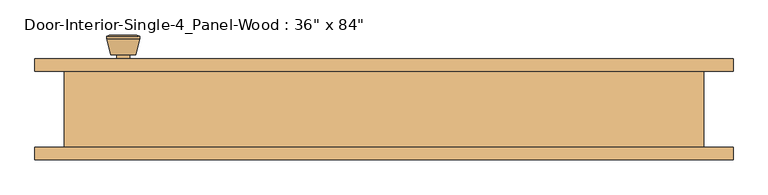
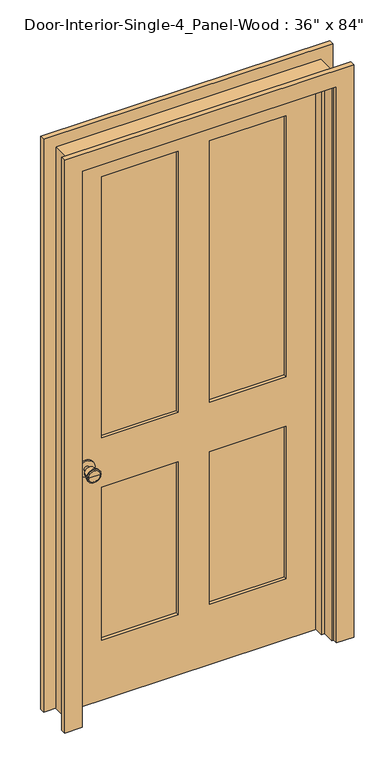
"""IFC4 building model written with IfcOpenShell, lengths in millimetres: door geometry."""

from ifc_helpers import new_model, si_unit, point, frame, frame_2d, origin, place, context, project, spatial, polyline, circle_curve, trimmed, segment, composite_curve, outline, extrude, faceted_brep, source, transform, mapped, element, save
from ifc_brep_helpers import plane_surface, cylinder_surface, revolved_surface, advanced_brep


def door_c2926031(model_context):
    return source(origin(), model_context, "Body", "SolidModel", [
        advanced_brep(
        [(-393.7, 13.05, 914.4), (-383.7, 13.05, 914.4), (-403.7, 13.05, 914.4), (-373.2241324, -35.95, 914.4), (-393.7, -35.95, 914.4), (-414.1758676, -35.95, 914.4), (-368.7, -34.1221319, 914.4), (-418.7, -34.1221319, 914.4), (-368.7, -30.6584537, 914.4), (-418.7, -30.6584537, 914.4), (-375.063764, -5.95, 914.4), (-412.336236, -5.95, 914.4), (-383.7, -5.95, 914.4), (-403.7, -5.95, 914.4)],
        [
            (0, 1),
            (1, 2, circle_curve(frame((-393.7, 13.05, 914.4), z_axis=(0.0, 1.0, 0.0), x_axis=(-1.0, 0.0, 0.0)), 10.0)),
            (2, 0),
            (2, 1, circle_curve(frame((-393.7, 13.05, 914.4), z_axis=(0.0, 1.0, 0.0), x_axis=(-1.0, 0.0, 0.0)), 10.0)),
            (3, 4),
            (4, 5),
            (5, 3, circle_curve(frame((-393.7, -35.95, 914.4), z_axis=(0.0, -1.0, 0.0), x_axis=(-1.0, 0.0, 0.0)), 20.4758676)),
            (3, 5, circle_curve(frame((-393.7, -35.95, 914.4), z_axis=(0.0, -1.0, 0.0), x_axis=(-1.0, 0.0, 0.0)), 20.4758676)),
            (6, 3),
            (5, 7),
            (7, 6, circle_curve(frame((-393.7, -34.1221319, 914.4), z_axis=(0.0, -1.0, 0.0), x_axis=(-1.0, 0.0, 0.0)), 25.0)),
            (6, 7, circle_curve(frame((-393.7, -34.1221319, 914.4), z_axis=(0.0, -1.0, 0.0), x_axis=(-1.0, 0.0, 0.0)), 25.0)),
            (8, 6),
            (7, 9),
            (9, 8, circle_curve(frame((-393.7, -30.6584537, 914.4), z_axis=(0.0, -1.0, 0.0), x_axis=(-1.0, 0.0, 0.0)), 25.0)),
            (8, 9, circle_curve(frame((-393.7, -30.6584537, 914.4), z_axis=(0.0, -1.0, 0.0), x_axis=(-1.0, 0.0, 0.0)), 25.0)),
            (10, 8),
            (9, 11),
            (11, 10, circle_curve(frame((-393.7, -5.95, 914.4), z_axis=(0.0, -1.0, 0.0), x_axis=(-1.0, 0.0, 0.0)), 18.636236)),
            (10, 11, circle_curve(frame((-393.7, -5.95, 914.4), z_axis=(0.0, -1.0, 0.0), x_axis=(-1.0, 0.0, 0.0)), 18.636236)),
            (12, 10),
            (11, 13),
            (13, 12, circle_curve(frame((-393.7, -5.95, 914.4), z_axis=(0.0, -1.0, 0.0), x_axis=(-1.0, 0.0, 0.0)), 10.0)),
            (12, 13, circle_curve(frame((-393.7, -5.95, 914.4), z_axis=(0.0, -1.0, 0.0), x_axis=(-1.0, 0.0, 0.0)), 10.0)),
            (1, 12),
            (13, 2),
        ],
        [
            plane_surface(frame((-393.7, 13.05, 914.4), z_axis=(0.0, 1.0, 0.0), x_axis=(-1.0, 0.0, 0.0))),
            plane_surface(frame((-393.7, -35.95, 914.4), z_axis=(0.0, -1.0, 0.0), x_axis=(-1.0, 0.0, 0.0))),
            revolved_surface(polyline([(-414.1758676, -35.95, 914.4), (-418.7, -34.1221319, 914.4)]), (-393.7, 13.05, 914.4), (0.0, 1.0, 0.0)),
            cylinder_surface(frame((-393.7, 13.05, 914.4), z_axis=(0.0, 1.0, 0.0), x_axis=(-1.0, 0.0, 0.0)), 25.0),
            revolved_surface(polyline([(-418.7, -30.6584537, 914.4), (-412.336236, -5.95, 914.4)]), (-393.7, 13.05, 914.4), (0.0, 1.0, 0.0)),
            plane_surface(frame((-393.7, -5.95, 914.4), z_axis=(0.0, 1.0, 0.0), x_axis=(-1.0, 0.0, 0.0))),
            cylinder_surface(frame((-393.7, 13.05, 914.4), z_axis=(0.0, 1.0, 0.0), x_axis=(-1.0, 0.0, 0.0)), 10.0),
        ],
        [
            (0, [[1, 2, 3]]),
            (0, [[-3, 4, -1]]),
            (1, [[5, 6, 7]]),
            (1, [[-6, -5, 8]]),
            (2, [[9, -7, 10, 11]]),
            (2, [[-10, -8, -9, 12]]),
            (3, [[13, -11, 14, 15]]),
            (3, [[-14, -12, -13, 16]]),
            (4, [[17, -15, 18, 19]]),
            (4, [[-18, -16, -17, 20]]),
            (5, [[21, -19, 22, 23]]),
            (5, [[-22, -20, -21, 24]]),
            (6, [[25, -23, 26, -2]]),
            (6, [[-26, -24, -25, -4]]),
        ],
    ),
        extrude(outline(composite_curve([segment(trimmed(circle_curve(frame_2d((914.4, -393.7)), 30.0), [point((914.4, -423.7))], [point((914.4, -363.7))], False, "CARTESIAN"), True, "CONTINUOUS"), segment(trimmed(circle_curve(frame_2d((914.4, -393.7)), 30.0), [point((914.4, -363.7))], [point((914.4, -423.7))], False, "CARTESIAN"), True, "CONTINUOUS")], self_intersect=False)), frame((0.0, 13.05, 0.0), z_axis=(0.0, 1.0, 0.0), x_axis=(0.0, 0.0, 1.0)), (0.0, 0.0, 1.0), 6.0),
        advanced_brep(
        [(-393.7, 59.975, 914.4), (-403.7, 59.975, 914.4), (-383.7, 59.975, 914.4), (-373.2241324, 108.975, 914.4), (-414.1758676, 108.975, 914.4), (-393.7, 108.975, 914.4), (-368.7, 107.1471319, 914.4), (-418.7, 107.1471319, 914.4), (-368.7, 103.6834537, 914.4), (-418.7, 103.6834537, 914.4), (-375.063764, 78.975, 914.4), (-412.336236, 78.975, 914.4), (-383.7, 78.975, 914.4), (-403.7, 78.975, 914.4)],
        [
            (0, 1),
            (1, 2, circle_curve(frame((-393.7, 59.975, 914.4), z_axis=(0.0, -1.0, 0.0), x_axis=(-1.0, 0.0, 0.0)), 10.0)),
            (2, 0),
            (2, 1, circle_curve(frame((-393.7, 59.975, 914.4), z_axis=(0.0, -1.0, 0.0), x_axis=(-1.0, 0.0, 0.0)), 10.0)),
            (3, 4, circle_curve(frame((-393.7, 108.975, 914.4), z_axis=(0.0, 1.0, 0.0), x_axis=(-1.0, 0.0, 0.0)), 20.4758676)),
            (4, 5),
            (5, 3),
            (4, 3, circle_curve(frame((-393.7, 108.975, 914.4), z_axis=(0.0, 1.0, 0.0), x_axis=(-1.0, 0.0, 0.0)), 20.4758676)),
            (6, 7, circle_curve(frame((-393.7, 107.1471319, 914.4), z_axis=(0.0, 1.0, 0.0), x_axis=(-1.0, 0.0, 0.0)), 25.0)),
            (7, 4),
            (3, 6),
            (7, 6, circle_curve(frame((-393.7, 107.1471319, 914.4), z_axis=(0.0, 1.0, 0.0), x_axis=(-1.0, 0.0, 0.0)), 25.0)),
            (8, 9, circle_curve(frame((-393.7, 103.6834537, 914.4), z_axis=(0.0, 1.0, 0.0), x_axis=(-1.0, 0.0, 0.0)), 25.0)),
            (9, 7),
            (6, 8),
            (9, 8, circle_curve(frame((-393.7, 103.6834537, 914.4), z_axis=(0.0, 1.0, 0.0), x_axis=(-1.0, 0.0, 0.0)), 25.0)),
            (10, 11, circle_curve(frame((-393.7, 78.975, 914.4), z_axis=(0.0, 1.0, 0.0), x_axis=(-1.0, 0.0, 0.0)), 18.636236)),
            (11, 9),
            (8, 10),
            (11, 10, circle_curve(frame((-393.7, 78.975, 914.4), z_axis=(0.0, 1.0, 0.0), x_axis=(-1.0, 0.0, 0.0)), 18.636236)),
            (12, 13, circle_curve(frame((-393.7, 78.975, 914.4), z_axis=(0.0, 1.0, 0.0), x_axis=(-1.0, 0.0, 0.0)), 10.0)),
            (13, 11),
            (10, 12),
            (13, 12, circle_curve(frame((-393.7, 78.975, 914.4), z_axis=(0.0, 1.0, 0.0), x_axis=(-1.0, 0.0, 0.0)), 10.0)),
            (1, 13),
            (12, 2),
        ],
        [
            plane_surface(frame((-393.7, 59.975, 914.4), z_axis=(0.0, -1.0, 0.0), x_axis=(-1.0, 0.0, 0.0))),
            plane_surface(frame((-393.7, 108.975, 914.4), z_axis=(0.0, 1.0, 0.0), x_axis=(-1.0, 0.0, 0.0))),
            revolved_surface(polyline([(-414.1758676, 108.975, 914.4), (-418.7, 107.1471319, 914.4)]), (-393.7, 59.975, 914.4), (0.0, -1.0, 0.0)),
            cylinder_surface(frame((-393.7, 59.975, 914.4), z_axis=(0.0, -1.0, 0.0), x_axis=(-1.0, 0.0, 0.0)), 25.0),
            revolved_surface(polyline([(-418.7, 103.6834537, 914.4), (-412.336236, 78.975, 914.4)]), (-393.7, 59.975, 914.4), (0.0, -1.0, 0.0)),
            plane_surface(frame((-393.7, 78.975, 914.4), z_axis=(0.0, -1.0, 0.0), x_axis=(-1.0, 0.0, 0.0))),
            cylinder_surface(frame((-393.7, 59.975, 914.4), z_axis=(0.0, -1.0, 0.0), x_axis=(-1.0, 0.0, 0.0)), 10.0),
        ],
        [
            (0, [[1, 2, 3]]),
            (0, [[-3, 4, -1]]),
            (1, [[5, 6, 7]]),
            (1, [[8, -7, -6]]),
            (2, [[9, 10, -5, 11]]),
            (2, [[12, -11, -8, -10]]),
            (3, [[13, 14, -9, 15]]),
            (3, [[16, -15, -12, -14]]),
            (4, [[17, 18, -13, 19]]),
            (4, [[20, -19, -16, -18]]),
            (5, [[21, 22, -17, 23]]),
            (5, [[24, -23, -20, -22]]),
            (6, [[-2, 25, -21, 26]]),
            (6, [[-4, -26, -24, -25]]),
        ],
    ),
        extrude(outline(composite_curve([segment(trimmed(circle_curve(frame_2d((914.4, -393.7)), 30.0), [point((914.4, -423.7))], [point((914.4, -363.7))], False, "CARTESIAN"), True, "CONTINUOUS"), segment(trimmed(circle_curve(frame_2d((914.4, -393.7)), 30.0), [point((914.4, -363.7))], [point((914.4, -423.7))], False, "CARTESIAN"), True, "CONTINUOUS")], self_intersect=False)), frame((0.0, 53.975, 0.0), z_axis=(0.0, 1.0, 0.0), x_axis=(0.0, 0.0, 1.0)), (0.0, 0.0, 1.0), 6.0),
        faceted_brep([(482.6, 53.975, 0.0), (482.6, -60.325, 0.0), (457.2, -60.325, 0.0), (457.2, -15.875, 0.0), (444.5, -15.875, 0.0), (444.5, 19.05, 0.0), (457.2, 19.05, 0.0), (457.2, 53.975, 0.0), (482.6, 53.975, 2159.0), (482.6, -60.325, 2159.0), (-482.6, -60.325, 2159.0), (-482.6, -60.325, 0.0), (-457.2, -60.325, 0.0), (-457.2, -60.325, 2133.6), (457.2, -60.325, 2133.6), (457.2, -15.875, 2133.6), (-457.2, -15.875, 2133.6), (-457.2, -15.875, 0.0), (-444.5, -15.875, 0.0), (-444.5, -15.875, 2120.9), (444.5, -15.875, 2120.9), (444.5, 19.05, 2120.9), (-444.5, 19.05, 2120.9), (-444.5, 19.05, 0.0), (-457.2, 19.05, 0.0), (-457.2, 19.05, 2133.6), (457.2, 19.05, 2133.6), (457.2, 53.975, 2133.6), (-457.2, 53.975, 2133.6), (-457.2, 53.975, 0.0), (-482.6, 53.975, 0.0), (-482.6, 53.975, 2159.0)], [[[0, 1, 2, 3, 4, 5, 6, 7]], [[1, 0, 8, 9]], [[2, 1, 9, 10, 11, 12, 13, 14]], [[3, 2, 14, 15]], [[4, 3, 15, 16, 17, 18, 19, 20]], [[5, 4, 20, 21]], [[6, 5, 21, 22, 23, 24, 25, 26]], [[7, 6, 26, 27]], [[0, 7, 27, 28, 29, 30, 31, 8]], [[9, 8, 31, 10]], [[15, 14, 13, 16]], [[21, 20, 19, 22]], [[27, 26, 25, 28]], [[30, 29, 24, 23, 18, 17, 12, 11]], [[10, 31, 30, 11]], [[16, 13, 12, 17]], [[22, 19, 18, 23]], [[28, 25, 24, 29]]]),
        extrude(outline(polyline([(2133.6, -457.2), (0.0, -457.2), (0.0, 457.2), (2133.6, 457.2), (2133.6, -457.2)]), holes=[polyline([(2014.5375, 57.15), (2014.5375, 336.55), (1009.65, 336.55), (1009.65, 57.15), (2014.5375, 57.15)]), polyline([(1009.65, -57.15), (1009.65, -336.55), (2014.5375, -336.55), (2014.5375, -57.15), (1009.65, -57.15)]), polyline([(819.15, 57.15), (819.15, 336.55), (231.775, 336.55), (231.775, 57.15), (819.15, 57.15)]), polyline([(231.775, -57.15), (231.775, -336.55), (819.15, -336.55), (819.15, -57.15), (231.775, -57.15)])]), frame((0.0, 19.05, 0.0), z_axis=(0.0, 1.0, 0.0), x_axis=(0.0, 0.0, 1.0)), (0.0, 0.0, 1.0), 34.925),
        extrude(outline(polyline([(336.55, 30.6916667), (57.15, 30.6916667), (57.15, 42.3333333), (336.55, 42.3333333), (336.55, 30.6916667)])), frame((0.0, 0.0, 1009.65), z_axis=(0.0, 0.0, 1.0), x_axis=(1.0, 0.0, 0.0)), (0.0, 0.0, 1.0), 1004.8875),
        extrude(outline(polyline([(-57.15, 30.6916667), (-336.55, 30.6916667), (-336.55, 42.3333333), (-57.15, 42.3333333), (-57.15, 30.6916667)])), frame((0.0, 0.0, 1009.65), z_axis=(0.0, 0.0, 1.0), x_axis=(1.0, 0.0, 0.0)), (0.0, 0.0, 1.0), 1004.8875),
        extrude(outline(polyline([(336.55, 30.6916667), (57.15, 30.6916667), (57.15, 42.3333333), (336.55, 42.3333333), (336.55, 30.6916667)])), frame((0.0, 0.0, 231.775), z_axis=(0.0, 0.0, 1.0), x_axis=(1.0, 0.0, 0.0)), (0.0, 0.0, 1.0), 587.375),
        extrude(outline(polyline([(-57.15, 30.6916667), (-336.55, 30.6916667), (-336.55, 42.3333333), (-57.15, 42.3333333), (-57.15, 30.6916667)])), frame((0.0, 0.0, 231.775), z_axis=(0.0, 0.0, 1.0), x_axis=(1.0, 0.0, 0.0)), (0.0, 0.0, 1.0), 587.375),
        extrude(outline(polyline([(0.0, 463.55), (0.0, 527.05), (2203.45, 527.05), (2203.45, -527.05), (0.0, -527.05), (0.0, -463.55), (2139.95, -463.55), (2139.95, 463.55), (0.0, 463.55)])), frame((0.0, 53.975, 0.0), z_axis=(0.0, 1.0, 0.0), x_axis=(0.0, 0.0, 1.0)), (0.0, 0.0, 1.0), 19.05),
        extrude(outline(polyline([(0.0, 463.55), (0.0, 527.05), (2203.45, 527.05), (2203.45, -527.05), (0.0, -527.05), (0.0, -463.55), (2139.95, -463.55), (2139.95, 463.55), (0.0, 463.55)])), frame((0.0, -79.375, 0.0), z_axis=(0.0, 1.0, 0.0), x_axis=(0.0, 0.0, 1.0)), (0.0, 0.0, 1.0), 19.05),
    ])


if __name__ == "__main__":
    model = new_model("IFC4")
    model_context = context("Model", 3, world=origin())
    ifc_project = project(units=[si_unit("LENGTHUNIT", "METRE", prefix="MILLI")], contexts=[model_context])
    site = spatial("IfcSite", under=ifc_project)
    building = spatial("IfcBuilding", under=site)
    placement = place(None, origin())
    door_shape = door_c2926031(model_context)
    element("IfcDoor", 1, ObjectType="Door-Interior-Single-4_Panel-Wood : 36\" x 84\"", at=placement, inside=building, context=model_context, shape_type="MappedRepresentation", body=[
        mapped(door_shape, transform((0.0, 0.0, 0.0), x_axis=(1.0, 0.0, 0.0), y_axis=(0.0, 1.0, 0.0), z_axis=(0.0, 0.0, 1.0))),
    ])
    save(model, "model.ifc")

# Revit data of these elements
# Type "Door-Interior-Single-4_Panel-Wood : 36\" x 84\""
#   Type Mark = "8"
#   Assembly Code = "C1020300"
#   Analytic Construction = "Wooden"
#   Top Rail = 0' - 4 11/16"
#   Thickness = 0' - 1 3/8"
#   Thermal Resistance (R) = 2.5876 (h·ft²·°F)/BTU
#   Swing Angle [instance default] = 90.00°
#   Stiles = 0' - 4 3/4"
#   Rough Width = 3' - 2"
#   Rough Height = 7' - 1"
#   Mullion = 0' - 4 1/2"
#   Lock Rail = 0' - 7 1/2"
#   Height = 7' - 0"
#   Width = 3' - 0"
#   Heat Transfer Coefficient (U) = 0.3865 BTU/(h·ft²·°F)
#   Bottom Rail = 0' - 9 1/8"
#   Trim Material = Cherry
#   Panel Material = Cherry
#   Frame Material = Cherry
#   Door Handle Material = Aluminum
#   Visual Light Transmittance = 0
#   Solar Heat Gain Coefficient = 0
#   Wall Closure = (empty or 0)
#   Function = (empty or 0)
# Element 1 (IfcDoor, "Door-Interior-Single-4_Panel-Wood : 36\" x 84\"")
#   Materials on its faces: "Cherry", "Aluminum"
# Materials
#   "Cherry": class "Wood", colour RGB 226 177 128, transparency 0, Description = "Prunus Serotina", Cost = 0
#   "Aluminum": class "Metal", colour RGB 247 247 247, transparency 0, Description = "Aluminum 6061", Cost = 0
